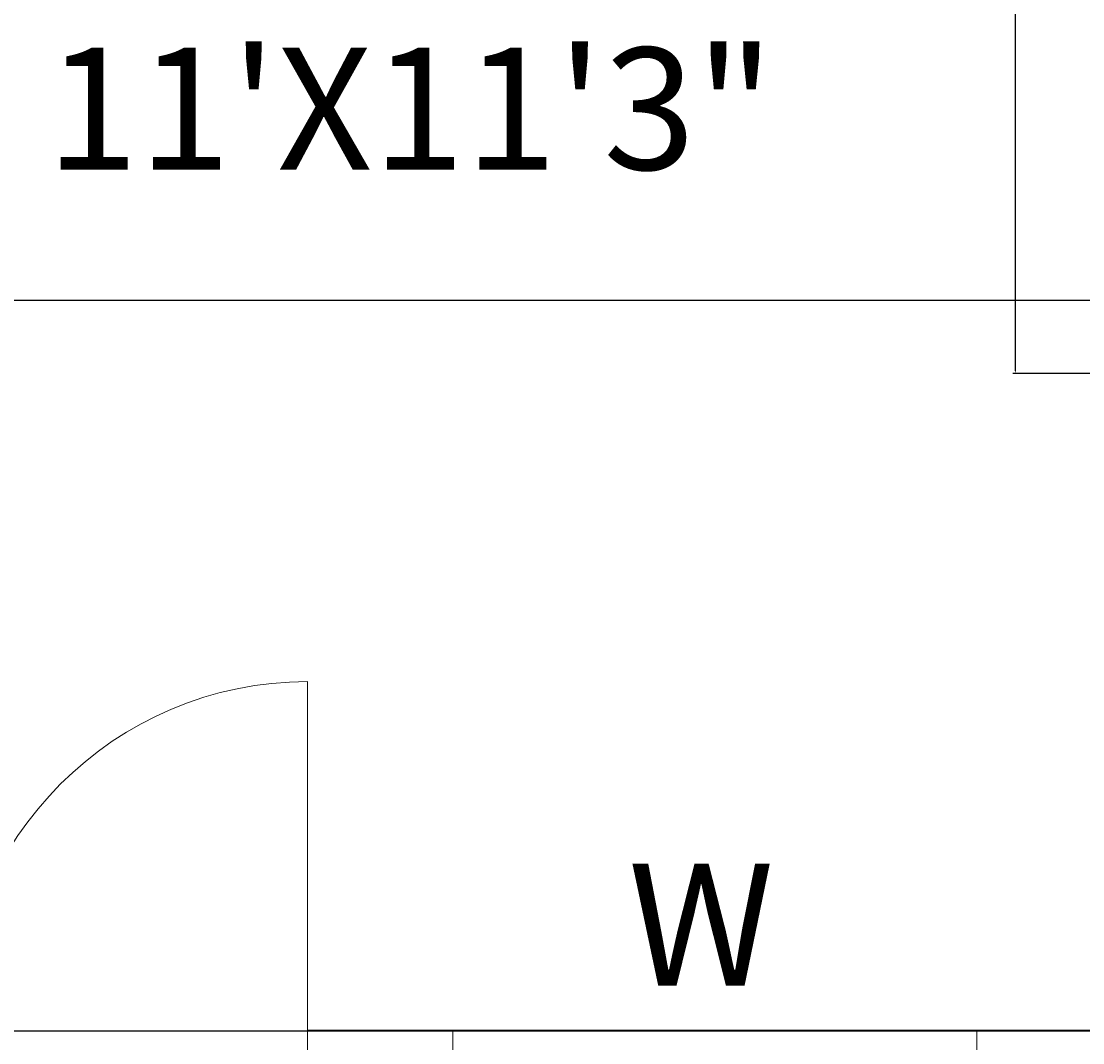
# Model space of a CAD drawing. Units: feet. Extents: x 1654 to 2985, y 1348 to 2230.
# Tile 35 of 53: x 2100 to 2173, y 1750 to 1821. Entities that reach past the tile are written whole.
import ezdxf

# ---------------------------------------------------------------- set-up
doc = ezdxf.new("R2010")
doc.units = ezdxf.units.FT
for name, color, linetype, lineweight in [('A-ANNO-DIMS', 2, 'Continuous', 18), ('A-ANNO-TEXT', 7, 'Continuous', 18), ('A-AREA-IDEN', 7, 'Continuous', 18), ('A-DOOR', 3, 'Continuous', 18), ('A-FLOR-STRS', 7, 'Continuous', 18), ('A-WALL', 7, 'Continuous', 35)]:
    doc.layers.add(name, color=color, linetype=linetype, lineweight=lineweight)
doc.styles.get("Standard").update_dxf_attribs({"font": 'arial.ttf'})
doc.dimstyles.get("Standard").update_dxf_attribs({"dimtxt": 0.18, "dimasz": 0.18, "dimexe": 0.18, "dimexo": 0.0625, "dimgap": 0.09, "dimtad": 0, "dimtih": 1, "dimtoh": 1, "dimdec": 4, "dimzin": 0, "dimdsep": 46, "dimtxsty": 'Standard', "dimcen": 0.09, "dimadec": 0, "dimazin": 0, "dimtfac": 1, "dimtdec": 4, "dimtofl": 0, "dimtmove": 0, "dimatfit": 3, "dimfxl": 1, "dimtolj": 1, "dimtzin": 0, "dimarcsym": 0})

# ---------------------------------------------------------------- blocks, each defined once
blk = doc.blocks.new('DOOR-ENTRY-PAIR')
for p, q in [((0, -9), (0, 24)), ((48, -9), (48, 24))]:
    blk.add_line(p, q)
for centre, start, end in [((0, 0), 0, 90), ((48, 0), 90, 180)]:
    blk.add_arc(centre, 24, start, end)
blk = doc.blocks.new('STAIR-RETURN')
for p, q in [((0, 186), (0, 135)), ((36, 186), (36, 0))]:
    blk.add_line(p, q)
blk = doc.blocks.new('*D38')
at = {"layer": 'A-ANNO-DIMS', "color": 0, "lineweight": -2, "transparency": 16777216}
for p, q in [((2176.839, 1850.733), (2168.575, 1850.733)), ((2168.755, 1850.553), (2168.755, 1823.764)), ((2168.755, 1796.609), (2168.755, 1823.398)), ((2176.839, 1796.429), (2168.575, 1796.429))]:
    blk.add_line(p, q, dxfattribs=at)
at = {"layer": 'A-ANNO-DIMS', "color": 0, "transparency": 16777216}
for points in [[(2168.725, 1850.553), (2168.785, 1850.553), (2168.755, 1850.733)], [(2168.725, 1796.609), (2168.785, 1796.609), (2168.755, 1796.429)]]:
    blk.add_solid(points, dxfattribs=at)
at = {"layer": 'Defpoints', "color": 0, "transparency": 16777216}
for p in [(2176.901, 1850.733), (2168.755, 1796.429), (2176.901, 1796.429)]:
    blk.add_point(p, dxfattribs=at)
at = {"layer": 'A-ANNO-DIMS', "color": 0, "transparency": 16777216, "insert": (2168.755, 1823.581), "char_height": 0.18, "attachment_point": 5}
blk.add_mtext('\\A1;SOFA 54 TYP.', dxfattribs=at)
blk = doc.blocks.new('*D80')
at = {"layer": 'A-ANNO-DIMS', "color": 0, "lineweight": -2, "transparency": 16777216}
for p, q in [((2070.092, 2039.192), (2070.092, 1534.075)), ((2202.092, 2039.192), (2202.092, 1534.075)), ((2070.272, 1534.255), (2135.813, 1534.255)), ((2201.912, 1534.255), (2136.372, 1534.255))]:
    blk.add_line(p, q, dxfattribs=at)
at = {"layer": 'A-ANNO-DIMS', "color": 0, "transparency": 16777216}
for points in [[(2070.272, 1534.285), (2070.272, 1534.225), (2070.092, 1534.255)], [(2201.912, 1534.285), (2201.912, 1534.225), (2202.092, 1534.255)]]:
    blk.add_solid(points, dxfattribs=at)
at = {"layer": 'Defpoints', "color": 0, "transparency": 16777216}
for p in [(2070.092, 2039.255), (2202.092, 2039.255), (2202.092, 1534.255)]:
    blk.add_point(p, dxfattribs=at)
at = {"layer": 'A-ANNO-DIMS', "color": 0, "transparency": 16777216, "insert": (2136.092, 1534.255), "char_height": 0.18, "attachment_point": 5}
blk.add_mtext('\\A1;132', dxfattribs=at)
blk = doc.blocks.new('*D91')
at = {"layer": 'A-ANNO-DIMS', "color": 0, "lineweight": -2, "transparency": 16777216}
for p, q in [((1852.155, 1801.468), (2242.272, 1801.468)), ((2242.092, 1801.288), (2242.092, 1776.544)), ((2242.092, 1751.435), (2242.092, 1776.18)), ((1852.155, 1751.255), (2242.272, 1751.255))]:
    blk.add_line(p, q, dxfattribs=at)
at = {"layer": 'A-ANNO-DIMS', "color": 0, "transparency": 16777216}
for points in [[(2242.062, 1801.288), (2242.122, 1801.288), (2242.092, 1801.468)], [(2242.062, 1751.435), (2242.122, 1751.435), (2242.092, 1751.255)]]:
    blk.add_solid(points, dxfattribs=at)
at = {"layer": 'Defpoints', "color": 0, "transparency": 16777216}
for p in [(1852.092, 1801.468), (2242.092, 1801.468), (1852.092, 1751.255)]:
    blk.add_point(p, dxfattribs=at)
at = {"layer": 'A-ANNO-DIMS', "color": 0, "transparency": 16777216, "insert": (2242.092, 1776.362), "char_height": 0.18, "attachment_point": 5}
blk.add_mtext('\\A1;50.21', dxfattribs=at)

msp = doc.modelspace()

# ---------------------------------------------------------------- linework, layer by layer
at = {"layer": 'A-WALL'}
msp.add_line((2202.0924, 1751.2549), (2120.0924, 1751.2549), dxfattribs=at)

# ---------------------------------------------------------------- block references
at = {"layer": 'A-DOOR'}
msp.add_blockref('DOOR-ENTRY-PAIR', (2072.0924, 1751.2549), dxfattribs=at)
at = {"layer": 'A-FLOR-STRS'}
msp.add_blockref('STAIR-RETURN', (2130.092, 1565.255), dxfattribs=at)

# ---------------------------------------------------------------- texts
at = {"layer": 'A-ANNO-TEXT'}
msp.add_text('W', height=8.3811, dxfattribs=at).set_placement((2142.1288, 1754.3563))
at = {"layer": 'A-AREA-IDEN'}
msp.add_text('11\'X11\'3"', height=8.38114, dxfattribs=at).set_placement((2102.1259, 1810.4431))

# ---------------------------------------------------------------- dimensions: what is measured, and where the dimension line sits
at = {"layer": 'A-ANNO-DIMS'}
dim = msp.add_linear_dim(base=(2202.0924, 1534.2549), p1=(2070.0924, 2039.2549), p2=(2202.0924, 2039.2549), dimstyle='Standard', override={"dimdec": 0, "dimlfac": 1, "dimrnd": 0, "dimzin": 0, "dimdsep": 46, "dimlunit": 2}, dxfattribs=at)
dim.commit()
dim.dimension.update_dxf_attribs({"geometry": '*D80', "text_midpoint": (2136.0924, 1534.2549)})
dim = msp.add_linear_dim(base=(2168.7554, 1796.4287), p1=(2176.9011, 1850.7334), p2=(2176.9011, 1796.4287), angle=270, text='SOFA <> TYP.', dimstyle='Standard', override={"dimdec": 0, "dimlfac": 1, "dimrnd": 0, "dimzin": 0, "dimdsep": 46, "dimlunit": 2}, dxfattribs=at)
dim.commit()
dim.dimension.update_dxf_attribs({"geometry": '*D38', "text_midpoint": (2168.7554, 1823.5811)})
dim = msp.add_linear_dim(base=(2242.0924, 1801.4683), p1=(1852.0924, 1751.2549), p2=(1852.0924, 1801.4683), angle=90, dimstyle='Standard', override={"dimdec": 2, "dimlfac": 1, "dimrnd": 0, "dimzin": 0, "dimdsep": 46, "dimlunit": 2}, dxfattribs=at)
dim.commit()
dim.dimension.update_dxf_attribs({"geometry": '*D91', "text_midpoint": (2242.0924, 1776.3616)})

doc.saveas('drawing.dxf')
